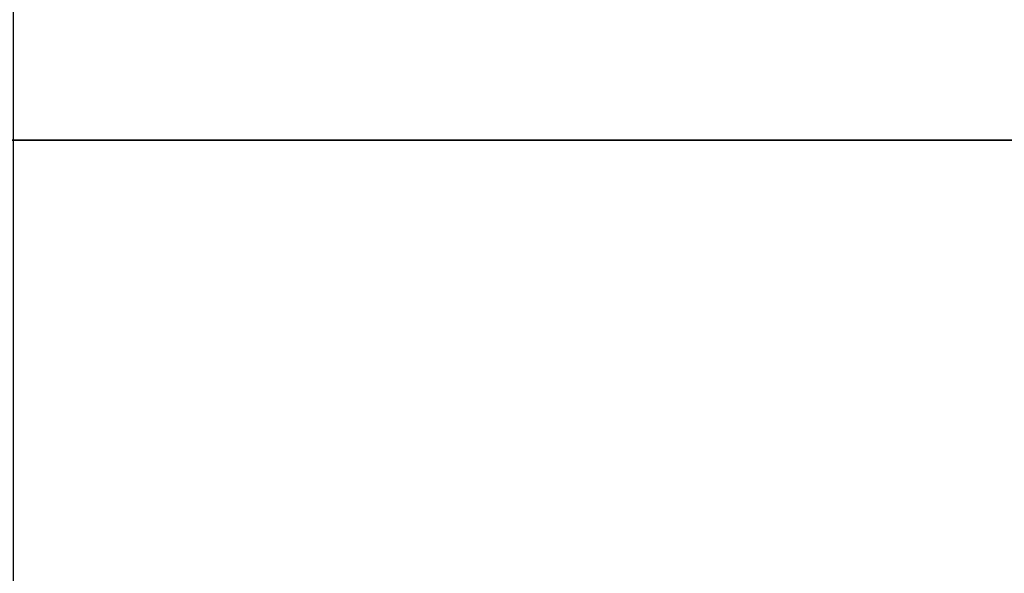
# Model space of a CAD drawing. Units: inches. Extents: x 3321 to 5237, y 11 to 1752.
# Tile 32 of 43: x 5059.68 to 5077.55, y 1426.48 to 1436.52. Entities that reach past the tile are written whole.
import ezdxf

# ---------------------------------------------------------------- set-up
doc = ezdxf.new("R2010")
doc.units = ezdxf.units.IN
doc.layers.add('A-ANNO-DIMS', color=2, linetype='Continuous', lineweight=18)
doc.layers.add('A-WALL', color=7, linetype='Continuous', lineweight=35)
doc.styles.get("Standard").update_dxf_attribs({"font": 'arial.ttf'})
doc.dimstyles.new('ISO-25', dxfattribs={"dimtxt": 9, "dimasz": 2.5, "dimexe": 1.25, "dimexo": 0.625, "dimtad": 1, "dimdec": 1, "dimlunit": 3, "dimtxsty": 'Standard', "dimcen": 2.5, "dimclrd": 4, "dimclre": 4, "dimclrt": 256, "dimadec": 0, "dimazin": 0, "dimtfac": 1, "dimtdec": 1, "dimtmove": 0, "dimatfit": 3, "dimfxl": 1, "dimarcsym": 0})

# ---------------------------------------------------------------- blocks, each defined once
blk = doc.blocks.new('*D194')
at = {"layer": 'A-ANNO-DIMS', "color": 4, "lineweight": -2, "transparency": 16777216}
for p, q in [((5037.321, 1452.516), (5037.321, 1436.712)), ((5121.084, 1452.516), (5121.084, 1436.712)), ((5039.821, 1437.962), (5118.584, 1437.962))]:
    blk.add_line(p, q, dxfattribs=at)
at = {"layer": 'A-ANNO-DIMS', "color": 4, "transparency": 16777216}
for points in [[(5039.821, 1438.379), (5039.821, 1437.545), (5037.321, 1437.962)], [(5118.584, 1438.379), (5118.584, 1437.545), (5121.084, 1437.962)]]:
    blk.add_solid(points, dxfattribs=at)
at = {"layer": 'Defpoints', "color": 0, "transparency": 16777216}
for p in [(5037.321, 1453.141), (5121.084, 1453.141), (5121.084, 1437.962)]:
    blk.add_point(p, dxfattribs=at)
at = {"layer": 'A-ANNO-DIMS', "transparency": 16777216, "insert": (5079.203, 1443.182), "char_height": 9, "attachment_point": 5}
blk.add_mtext('7\'-0" TYP.', dxfattribs=at)
blk = doc.blocks.new('*D199')
at = {"layer": 'A-ANNO-DIMS', "color": 4, "lineweight": -2, "transparency": 16777216}
for p, q in [((5059.569, 1379.636), (5059.569, 1473.411)), ((5060.444, 1379.636), (5058.319, 1379.636)), ((5059.569, 1372.136), (5059.569, 1377.136)), ((5060.444, 1369.636), (5058.319, 1369.636))]:
    blk.add_line(p, q, dxfattribs=at)
at = {"layer": 'A-ANNO-DIMS', "color": 4, "transparency": 16777216}
for points in [[(5059.153, 1377.136), (5059.986, 1377.136), (5059.569, 1379.636)], [(5059.153, 1372.136), (5059.986, 1372.136), (5059.569, 1369.636)]]:
    blk.add_solid(points, dxfattribs=at)
at = {"layer": 'Defpoints', "color": 0, "transparency": 16777216}
for p in [(5059.569, 1379.636), (5061.069, 1379.636), (5061.069, 1369.636)]:
    blk.add_point(p, dxfattribs=at)
at = {"layer": 'A-ANNO-DIMS', "transparency": 16777216, "insert": (5054.349, 1427.773), "char_height": 9, "attachment_point": 5, "rotation": 90}
blk.add_mtext('TAP 0\'-10" TYP.', dxfattribs=at)

msp = doc.modelspace()

# ---------------------------------------------------------------- linework, layer by layer
at = {"layer": 'A-WALL'}
msp.add_line((5001.084, 1434.339), (5087.084, 1434.339), dxfattribs=at)

# ---------------------------------------------------------------- dimensions: what is measured, and where the dimension line sits
at = {"layer": 'A-ANNO-DIMS'}
dim = msp.add_linear_dim(base=(5059.569, 1379.636), p1=(5061.069, 1369.636), p2=(5061.069, 1379.636), angle=90, text='TAP <> TYP.', dimstyle='ISO-25', override={"dimdec": 1, "dimlfac": 1, "dimrnd": 0, "dimzin": 1, "dimdsep": 46, "dimlunit": 4, "dimfrac": 2}, dxfattribs=at)
dim.commit()
dim.dimension.update_dxf_attribs({"geometry": '*D199', "text_midpoint": (5054.349, 1427.773)})
dim = msp.add_linear_dim(base=(5121.084, 1437.962), p1=(5037.321, 1453.141), p2=(5121.084, 1453.141), text='<> TYP.', dimstyle='ISO-25', override={"dimdec": 1, "dimlfac": 1, "dimrnd": 0, "dimzin": 1, "dimdsep": 46, "dimlunit": 4, "dimfrac": 2}, dxfattribs=at)
dim.commit()
dim.dimension.update_dxf_attribs({"geometry": '*D194', "text_midpoint": (5079.203, 1443.182)})

doc.saveas('drawing.dxf')
